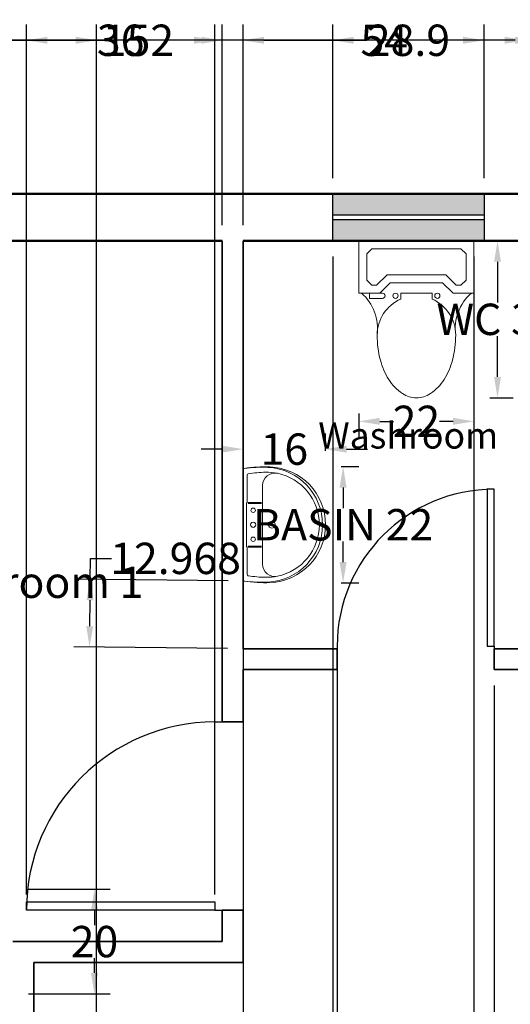
# Model space of a CAD drawing. Units: inches. Extents: x -1285 to -837, y -84 to 552.
# Tile 7 of 10: x -1131 to -1037, y 364 to 552. Entities that reach past the tile are written whole.
import ezdxf

# ---------------------------------------------------------------- set-up
doc = ezdxf.new("R2010")
doc.units = ezdxf.units.IN
doc.header["$MEASUREMENT"] = 0
for name, color, linetype, lineweight in [('A-ANNO-DIMS', 2, 'Continuous', 18), ('A-AREA-IDEN', 7, 'Continuous', 25), ('A-GLAZ-VENT-PATT', 130, 'Continuous', 13), ('Commode', 60, 'Continuous', 18), ('Doors', 34, 'Continuous', 25), ('Inner Wall', 202, 'Continuous', 35), ('Outer Wall', 12, 'Continuous', 50), ('Sink', 33, 'Continuous', 18), ('Ventilators', 130, 'Continuous', 25)]:
    doc.layers.add(name, color=color, linetype=linetype, lineweight=lineweight)
doc.styles.get("Standard").update_dxf_attribs({"font": 'arial.ttf'})
doc.dimstyles.get("Standard").update_dxf_attribs({"dimtxt": 6, "dimasz": 4, "dimexe": 3, "dimexo": 3, "dimgap": 0.09, "dimtad": 0, "dimtih": 1, "dimtoh": 1, "dimdec": 1, "dimzin": 0, "dimdsep": 46, "dimlunit": 3, "dimtxsty": 'Standard', "dimcen": 0.09, "dimadec": 0, "dimazin": 0, "dimtfac": 1, "dimtdec": 1, "dimtofl": 0, "dimtmove": 0, "dimatfit": 3, "dimfxl": 1, "dimtolj": 1, "dimtzin": 0, "dimarcsym": 0})

# ---------------------------------------------------------------- blocks, each defined once
blk = doc.blocks.new('B1')
at = {"color": 0}
for p, q in [((-342.1, -28), (-155.1, -28)), ((-153.6, -35.9), (-153.6, -126.6)), ((-147.1, -24), (-0.5, -24)), ((-147.1, -35.9), (-147.1, -126.6)), ((147.1, -24), (-0.5, -24)), ((147.1, -35.9), (147.1, -126.6)), ((153.6, -35.9), (153.6, -126.6)), ((342.1, -28), (155.1, -28)), ((-0.5, -135), (-272, -135)), ((-0.5, -135), (272.1, -135))]:
    blk.add_line(p, q, dxfattribs=at)
blk.add_lwpolyline([(0, -570, -0.403574), (-399.2, -186.1, -0.04955), (-388.9, -8.4, -0.368901), (-379, 0), (0, 0), (379.1, 0, -0.368901), (388.9, -8.4, -0.04955), (399.3, -186.1, -0.40261)], format="xyb", close=True, dxfattribs=at)
for centre in [(-100.5, -70), (100.6, -70)]:
    blk.add_circle(centre, 15, dxfattribs=at)
for centre, radius, start, end in [((502.9, -129.4), 900, 172.27277, 182.73185), ((437.5, -165.7), 800, 170.69697, 179.27367), ((-342.1, -38), 10, 90, 170.69697), ((-155.1, -24), 4, 270, 323.1301), ((-147.1, -30), 6, 90, 143.1301), ((-0.5, -70), 17.5, 90, 270), ((-0.5, -70), 17.5, 270, 90), ((147.1, -30), 6, 36.8699, 90), ((155.1, -24), 4, 216.8699, 270), ((342.1, -38), 10, 9.30303, 90), ((-437.5, -165.7), 800, 0.72633, 9.30303), ((-502.9, -129.4), 900, 357.26815, 7.72723), ((-272, -220), 85, 90, 191.45253), ((272.1, -220), 85, 348.54747, 90), ((-0.5, -153), 396, 182.79964, 270.07706), ((-0.5, -165), 362, 178.50683, 191.45253), ((0, -200), 23, 90, 270), ((-0.4, -152), 397, 270.055, 357.0633), ((0, -200), 23, 270, 90), ((0.6, -165), 362, 348.54747, 1.49317), ((-0.5, -165), 362, 191.45253, 270.0843), ((-0.4, -163.8), 363.2, 270.06445, 348.39326)]:
    blk.add_arc(centre, radius, start, end, dxfattribs=at)
blk = doc.blocks.new('A$C5EF6120A')
at = {"linetype": 'ByBlock'}
for p, q in [((0, 0.762), (0, 0.508)), ((0, 0.762), (0.5588, 0.762)), ((0.0381, 0.6985), (0.0635, 0.7239)), ((0.0635, 0.7239), (0.4953, 0.7239)), ((0.4953, 0.7239), (0.5207, 0.6985)), ((0.5588, 0.762), (0.5588, 0.508)), ((0.0381, 0.6985), (0.0381, 0.5715)), ((0.5207, 0.6985), (0.5207, 0.5715)), ((0.1366, 0.5969), (0.0858, 0.5461)), ((0.1366, 0.5969), (0.4222, 0.5969)), ((0.4222, 0.5969), (0.473, 0.5461)), ((0.0635, 0.5461), (0.0381, 0.5715)), ((0.0635, 0.5461), (0.0858, 0.5461)), ((0.1524, 0.5588), (0.1016, 0.508)), ((0.1524, 0.5588), (0.4064, 0.5588)), ((0.4064, 0.5588), (0.4572, 0.508)), ((0.4953, 0.5461), (0.473, 0.5461)), ((0.5207, 0.5715), (0.4953, 0.5461)), ((0, 0.508), (0.1016, 0.508)), ((0.0508, 0.508), (0.0508, 0.4826)), ((0.0508, 0.4826), (0.1143, 0.4826)), ((0.1143, 0.508), (0.1016, 0.508)), ((0.2032, 0.508), (0.2032, 0.4794)), ((0.3556, 0.508), (0.2032, 0.508)), ((0.3556, 0.508), (0.3556, 0.4794)), ((0.5588, 0.508), (0.4572, 0.508))]:
    blk.add_line(p, q, dxfattribs=at)
blk.add_lwpolyline([(0.0889, 0.3048, 0.063415), (0.1044, 0.183, 0.076468), (0.1447, 0.0893, 0.107136), (0.2118, 0.0204, 0.147373), (0.2794, 0, 0.147373), (0.347, 0.0204, 0.107136), (0.4141, 0.0893, 0.076468), (0.4544, 0.183, 0.063415), (0.4699, 0.3048, 0.063415)], format="xyb", dxfattribs=at)
for centre in [(0.1778, 0.4953), (0.381, 0.4953)]:
    blk.add_circle(centre, 0.0127, dxfattribs=at)
for centre, radius, start, end in [((-0.1375, 0.3358), 0.2285, 352.2011, 48.911), ((0.2794, 0.3048), 0.1905, 113.5782, 180), ((0.1143, 0.4953), 0.0127, 270, 90), ((0.2794, 0.3048), 0.1905, 0, 66.4218), ((0.6963, 0.3358), 0.2285, 131.089, 187.7989)]:
    blk.add_arc(centre, radius, start, end, dxfattribs=at)
blk = doc.blocks.new('*U3')
for p, q in [((0, 0), (0, -6)), ((40, 0), (40, -6))]:
    blk.add_line(p, q)
blk.add_lwpolyline([(0, 0), (0, 40), (1.75, 40), (1.75, 0)], close=True)
blk.add_arc((0, 0), 40, 0, 90)
blk = doc.blocks.new('*U16')
for p, q in [((0, 0), (0, -6)), ((-40, 0), (-40, -6))]:
    blk.add_line(p, q)
blk.add_lwpolyline([(0, 0), (0, 40), (-1.75, 40), (-1.75, 0)], close=True)
blk.add_arc((0, 0), 40, 90, 180)
blk = doc.blocks.new('*D37')
at = {"layer": 'A-ANNO-DIMS', "color": 0, "lineweight": -2, "transparency": 16777216}
for p, q in [((-1041.37, 509.94), (-1036.87, 509.94)), ((-1039.87, 505.94), (-1039.87, 498.13)), ((-1039.87, 483.93), (-1039.87, 491.74)), ((-1041.37, 479.93), (-1036.87, 479.93))]:
    blk.add_line(p, q, dxfattribs=at)
at = {"layer": 'A-ANNO-DIMS', "color": 0, "transparency": 16777216}
for points in [[(-1040.54, 505.94), (-1039.2, 505.94), (-1039.87, 509.94)], [(-1040.54, 483.93), (-1039.2, 483.93), (-1039.87, 479.93)]]:
    blk.add_solid(points, dxfattribs=at)
at = {"layer": 'Defpoints', "color": 0, "transparency": 16777216}
for p in [(-1044.37, 509.94), (-1039.87, 509.94), (-1044.37, 479.93)]:
    blk.add_point(p, dxfattribs=at)
at = {"layer": 'A-ANNO-DIMS', "color": 0, "transparency": 16777216, "insert": (-1039.87, 494.93), "char_height": 6, "attachment_point": 5}
blk.add_mtext('\\A1;WC 30', dxfattribs=at)
blk = doc.blocks.new('*D38')
at = {"layer": 'A-ANNO-DIMS', "color": 0, "lineweight": -2, "transparency": 16777216}
for p, q in [((-1066.38, 476.93), (-1066.38, 472.42)), ((-1044.37, 476.93), (-1044.37, 472.42)), ((-1062.38, 475.42), (-1059.78, 475.42)), ((-1048.37, 475.42), (-1050.97, 475.42))]:
    blk.add_line(p, q, dxfattribs=at)
at = {"layer": 'A-ANNO-DIMS', "color": 0, "transparency": 16777216}
for points in [[(-1062.38, 476.09), (-1062.38, 474.76), (-1066.38, 475.42)], [(-1048.37, 476.09), (-1048.37, 474.76), (-1044.37, 475.42)]]:
    blk.add_solid(points, dxfattribs=at)
at = {"layer": 'Defpoints', "color": 0, "transparency": 16777216}
for p in [(-1066.38, 479.93), (-1044.37, 479.93), (-1044.37, 475.42)]:
    blk.add_point(p, dxfattribs=at)
at = {"layer": 'A-ANNO-DIMS', "color": 0, "transparency": 16777216, "insert": (-1055.38, 475.42), "char_height": 6, "attachment_point": 5}
blk.add_mtext('\\A1;22', dxfattribs=at)
blk = doc.blocks.new('*D41')
at = {"layer": 'A-ANNO-DIMS', "color": 0, "lineweight": -2, "transparency": 16777216}
for p, q in [((-1069.74, 466.77), (-1066.4, 466.77)), ((-1069.4, 462.77), (-1069.4, 458.84)), ((-1069.4, 448.52), (-1069.4, 452.45)), ((-1069.74, 444.52), (-1066.4, 444.52))]:
    blk.add_line(p, q, dxfattribs=at)
at = {"layer": 'A-ANNO-DIMS', "color": 0, "transparency": 16777216}
for points in [[(-1070.07, 462.77), (-1068.73, 462.77), (-1069.4, 466.77)], [(-1070.07, 448.52), (-1068.73, 448.52), (-1069.4, 444.52)]]:
    blk.add_solid(points, dxfattribs=at)
at = {"layer": 'Defpoints', "color": 0, "transparency": 16777216}
for p in [(-1072.74, 466.77), (-1069.4, 466.77), (-1072.74, 444.52)]:
    blk.add_point(p, dxfattribs=at)
at = {"layer": 'A-ANNO-DIMS', "color": 0, "transparency": 16777216, "insert": (-1069.4, 455.65), "char_height": 6, "attachment_point": 5}
blk.add_mtext('\\A1;BASIN 22', dxfattribs=at)
blk = doc.blocks.new('*D42')
at = {"layer": 'A-ANNO-DIMS', "color": 0, "lineweight": -2, "transparency": 16777216}
for p, q in [((-1088.53, 469.77), (-1088.53, 473.11)), ((-1072.74, 469.77), (-1072.74, 473.11)), ((-1092.53, 470.11), (-1096.53, 470.11)), ((-1068.74, 470.11), (-1064.74, 470.11))]:
    blk.add_line(p, q, dxfattribs=at)
at = {"layer": 'A-ANNO-DIMS', "color": 0, "transparency": 16777216}
for points in [[(-1092.53, 470.77), (-1092.53, 469.44), (-1088.53, 470.11)], [(-1068.74, 470.77), (-1068.74, 469.44), (-1072.74, 470.11)]]:
    blk.add_solid(points, dxfattribs=at)
at = {"layer": 'Defpoints', "color": 0, "transparency": 16777216}
for p in [(-1088.53, 470.11), (-1088.53, 466.77), (-1072.74, 466.77)]:
    blk.add_point(p, dxfattribs=at)
at = {"layer": 'A-ANNO-DIMS', "color": 0, "transparency": 16777216, "insert": (-1080.63, 470.11), "char_height": 6, "attachment_point": 5}
blk.add_mtext('\\A1;16', dxfattribs=at)
blk = doc.blocks.new('*D60')
at = {"layer": 'A-ANNO-DIMS', "color": 0, "lineweight": -2, "transparency": 16777216}
for p, q in [((-1129.53, 385.94), (-1113.93, 385.94)), ((-1116.93, 381.94), (-1116.93, 379.09)), ((-1116.93, 369.94), (-1116.93, 372.79)), ((-1129.53, 365.94), (-1113.93, 365.94))]:
    blk.add_line(p, q, dxfattribs=at)
at = {"layer": 'A-ANNO-DIMS', "color": 0, "transparency": 16777216}
for points in [[(-1117.6, 381.94), (-1116.26, 381.94), (-1116.93, 385.94)], [(-1117.6, 369.94), (-1116.26, 369.94), (-1116.93, 365.94)]]:
    blk.add_solid(points, dxfattribs=at)
at = {"layer": 'Defpoints', "color": 0, "transparency": 16777216}
for p in [(-1132.53, 385.94), (-1116.93, 385.94), (-1132.53, 365.94)]:
    blk.add_point(p, dxfattribs=at)
at = {"layer": 'A-ANNO-DIMS', "color": 0, "transparency": 16777216, "insert": (-1116.93, 375.94), "char_height": 6, "attachment_point": 5}
blk.add_mtext('\\A1;20', dxfattribs=at)
blk = doc.blocks.new('*D71')
at = {"layer": 'A-ANNO-DIMS', "color": 0, "lineweight": -2, "transparency": 16777216}
for p, q in [((-1236.53, 512.94), (-1236.53, 551.29)), ((-1092.53, 512.94), (-1092.53, 551.29)), ((-1232.53, 548.29), (-1170.95, 548.29)), ((-1096.53, 548.29), (-1158.11, 548.29))]:
    blk.add_line(p, q, dxfattribs=at)
at = {"layer": 'A-ANNO-DIMS', "color": 0, "transparency": 16777216}
for points in [[(-1232.53, 548.96), (-1232.53, 547.62), (-1236.53, 548.29)], [(-1096.53, 548.96), (-1096.53, 547.62), (-1092.53, 548.29)]]:
    blk.add_solid(points, dxfattribs=at)
at = {"layer": 'Defpoints', "color": 0, "transparency": 16777216}
for p in [(-1092.53, 548.29), (-1236.53, 509.94), (-1092.53, 509.94)]:
    blk.add_point(p, dxfattribs=at)
at = {"layer": 'A-ANNO-DIMS', "color": 0, "transparency": 16777216, "insert": (-1164.53, 548.29), "char_height": 6, "attachment_point": 5}
blk.add_mtext('\\A1;144', dxfattribs=at)
blk = doc.blocks.new('*D72')
at = {"layer": 'A-ANNO-DIMS', "color": 0, "lineweight": -2, "transparency": 16777216}
for p, q in [((-1088.53, 512.94), (-1088.53, 551.29)), ((-1034.53, 512.94), (-1034.53, 551.29)), ((-1084.53, 548.29), (-1065.9, 548.29)), ((-1038.53, 548.29), (-1057.15, 548.29))]:
    blk.add_line(p, q, dxfattribs=at)
at = {"layer": 'A-ANNO-DIMS', "color": 0, "transparency": 16777216}
for points in [[(-1084.53, 548.96), (-1084.53, 547.62), (-1088.53, 548.29)], [(-1038.53, 548.96), (-1038.53, 547.62), (-1034.53, 548.29)]]:
    blk.add_solid(points, dxfattribs=at)
at = {"layer": 'Defpoints', "color": 0, "transparency": 16777216}
for p in [(-1034.53, 548.29), (-1088.53, 509.94), (-1034.53, 509.94)]:
    blk.add_point(p, dxfattribs=at)
at = {"layer": 'A-ANNO-DIMS', "color": 0, "transparency": 16777216, "insert": (-1061.53, 548.29), "char_height": 6, "attachment_point": 5}
blk.add_mtext('\\A1;54', dxfattribs=at)
blk = doc.blocks.new('*D78')
at = {"layer": 'A-ANNO-DIMS', "color": 0, "lineweight": -2, "transparency": 16777216}
for p, q in [((-1236.53, 162.94), (-1236.53, 551.29)), ((-1116.53, 162.94), (-1116.53, 551.29)), ((-1232.53, 548.29), (-1182.96, 548.29)), ((-1120.53, 548.29), (-1170.1, 548.29))]:
    blk.add_line(p, q, dxfattribs=at)
at = {"layer": 'A-ANNO-DIMS', "color": 0, "transparency": 16777216}
for points in [[(-1232.53, 548.96), (-1232.53, 547.62), (-1236.53, 548.29)], [(-1120.53, 548.96), (-1120.53, 547.62), (-1116.53, 548.29)]]:
    blk.add_solid(points, dxfattribs=at)
at = {"layer": 'Defpoints', "color": 0, "transparency": 16777216}
for p in [(-1116.53, 548.29), (-1236.53, 159.94), (-1116.53, 159.94)]:
    blk.add_point(p, dxfattribs=at)
at = {"layer": 'A-ANNO-DIMS', "color": 0, "transparency": 16777216, "insert": (-1176.53, 548.29), "char_height": 6, "attachment_point": 5}
blk.add_mtext('\\A1;120', dxfattribs=at)
blk = doc.blocks.new('*D80')
at = {"layer": 'A-ANNO-DIMS', "color": 0, "lineweight": -2, "transparency": 16777216}
for p, q in [((-1184.53, -13.66), (-1184.53, 551.29)), ((-1032.53, -13.66), (-1032.53, 551.29)), ((-1180.53, 548.29), (-1114.94, 548.29)), ((-1036.53, 548.29), (-1102.12, 548.29))]:
    blk.add_line(p, q, dxfattribs=at)
at = {"layer": 'A-ANNO-DIMS', "color": 0, "transparency": 16777216}
for points in [[(-1180.53, 548.96), (-1180.53, 547.62), (-1184.53, 548.29)], [(-1036.53, 548.96), (-1036.53, 547.62), (-1032.53, 548.29)]]:
    blk.add_solid(points, dxfattribs=at)
at = {"layer": 'Defpoints', "color": 0, "transparency": 16777216}
for p in [(-1032.53, 548.29), (-1184.53, -16.66), (-1032.53, -16.66)]:
    blk.add_point(p, dxfattribs=at)
at = {"layer": 'A-ANNO-DIMS', "color": 0, "transparency": 16777216, "insert": (-1108.53, 548.29), "char_height": 6, "attachment_point": 5}
blk.add_mtext('\\A1;152', dxfattribs=at)
blk = doc.blocks.new('*D87')
at = {"layer": 'A-ANNO-DIMS', "color": 0, "lineweight": -2, "transparency": 16777216}
for p, q in [((-1070.53, 424.94), (-1070.53, -83.53)), ((-1040.53, 424.94), (-1040.53, -83.53)), ((-1066.53, -80.53), (-1059.9, -80.53)), ((-1044.53, -80.53), (-1051.15, -80.53))]:
    blk.add_line(p, q, dxfattribs=at)
at = {"layer": 'A-ANNO-DIMS', "color": 0, "transparency": 16777216}
for points in [[(-1066.53, -79.86), (-1066.53, -81.2), (-1070.53, -80.53)], [(-1044.53, -79.86), (-1044.53, -81.2), (-1040.53, -80.53)]]:
    blk.add_solid(points, dxfattribs=at)
at = {"layer": 'Defpoints', "color": 0, "transparency": 16777216}
for p in [(-1070.53, 427.94), (-1040.53, 427.94), (-1040.53, -80.53)]:
    blk.add_point(p, dxfattribs=at)
at = {"layer": 'A-ANNO-DIMS', "color": 0, "transparency": 16777216, "insert": (-1055.53, -80.53), "char_height": 6, "attachment_point": 5}
blk.add_mtext('\\A1;30', dxfattribs=at)
blk = doc.blocks.new('*D89')
at = {"layer": 'A-ANNO-DIMS', "color": 0, "lineweight": -2, "transparency": 16777216}
for p, q in [((-1071.35, 521.94), (-1071.35, 551.29)), ((-1042.45, 521.94), (-1042.45, 551.29)), ((-1067.35, 548.29), (-1064.84, 548.29)), ((-1046.45, 548.29), (-1048.96, 548.29))]:
    blk.add_line(p, q, dxfattribs=at)
at = {"layer": 'A-ANNO-DIMS', "color": 0, "transparency": 16777216}
for points in [[(-1067.35, 548.96), (-1067.35, 547.62), (-1071.35, 548.29)], [(-1046.45, 548.96), (-1046.45, 547.62), (-1042.45, 548.29)]]:
    blk.add_solid(points, dxfattribs=at)
at = {"layer": 'Defpoints', "color": 0, "transparency": 16777216}
for p in [(-1042.45, 548.29), (-1071.35, 518.94), (-1042.45, 518.94)]:
    blk.add_point(p, dxfattribs=at)
at = {"layer": 'A-ANNO-DIMS', "color": 0, "transparency": 16777216, "insert": (-1056.9, 548.29), "char_height": 6, "attachment_point": 5}
blk.add_mtext('\\A1;28.9', dxfattribs=at)
blk = doc.blocks.new('*D90')
at = {"layer": 'A-ANNO-DIMS', "color": 0, "lineweight": -2, "transparency": 16777216}
for p, q in [((-1129.93, 384.94), (-1129.93, 551.29)), ((-1093.93, 384.94), (-1093.93, 551.29)), ((-1125.93, 548.29), (-1116.31, 548.29)), ((-1097.93, 548.29), (-1107.55, 548.29))]:
    blk.add_line(p, q, dxfattribs=at)
at = {"layer": 'A-ANNO-DIMS', "color": 0, "transparency": 16777216}
for points in [[(-1125.93, 548.96), (-1125.93, 547.62), (-1129.93, 548.29)], [(-1097.93, 548.96), (-1097.93, 547.62), (-1093.93, 548.29)]]:
    blk.add_solid(points, dxfattribs=at)
at = {"layer": 'Defpoints', "color": 0, "transparency": 16777216}
for p in [(-1093.93, 548.29), (-1129.93, 381.94), (-1093.93, 381.94)]:
    blk.add_point(p, dxfattribs=at)
at = {"layer": 'A-ANNO-DIMS', "color": 0, "transparency": 16777216, "insert": (-1111.93, 548.29), "char_height": 6, "attachment_point": 5}
blk.add_mtext('\\A1;36', dxfattribs=at)
blk = doc.blocks.new('*D103')
at = {"layer": 'A-ANNO-DIMS', "color": 0, "lineweight": -2, "transparency": 16777216}
for p, q in [((-1088.53, 506.94), (-1088.53, -83.53)), ((-1071.35, 506.94), (-1071.35, -83.53)), ((-1084.53, -80.53), (-1075.35, -80.53)), ((-1071.35, -80.53), (-1067.35, -80.53))]:
    blk.add_line(p, q, dxfattribs=at)
at = {"layer": 'A-ANNO-DIMS', "color": 0, "transparency": 16777216}
for points in [[(-1084.53, -79.86), (-1084.53, -81.2), (-1088.53, -80.53)], [(-1075.35, -79.86), (-1075.35, -81.2), (-1071.35, -80.53)]]:
    blk.add_solid(points, dxfattribs=at)
at = {"layer": 'Defpoints', "color": 0, "transparency": 16777216}
for p in [(-1088.53, 509.94), (-1071.35, 509.94), (-1071.35, -80.53)]:
    blk.add_point(p, dxfattribs=at)
at = {"layer": 'A-ANNO-DIMS', "color": 0, "transparency": 16777216, "insert": (-1057.41, -80.53), "char_height": 6, "attachment_point": 5}
blk.add_mtext('\\A1;17.18', dxfattribs=at)
blk = doc.blocks.new('*D104')
at = {"layer": 'A-ANNO-DIMS', "color": 0, "lineweight": -2, "transparency": 16777216}
for p, q in [((-1044.37, 506.94), (-1044.37, -83.53)), ((-1034.53, 506.94), (-1034.53, -83.53)), ((-1040.37, -80.53), (-1038.53, -80.53)), ((-1034.53, -80.53), (-1030.53, -80.53))]:
    blk.add_line(p, q, dxfattribs=at)
at = {"layer": 'A-ANNO-DIMS', "color": 0, "transparency": 16777216}
for points in [[(-1040.37, -79.86), (-1040.37, -81.2), (-1044.37, -80.53)], [(-1038.53, -79.86), (-1038.53, -81.2), (-1034.53, -80.53)]]:
    blk.add_solid(points, dxfattribs=at)
at = {"layer": 'Defpoints', "color": 0, "transparency": 16777216}
for p in [(-1044.37, 509.94), (-1034.53, 509.94), (-1034.53, -80.53)]:
    blk.add_point(p, dxfattribs=at)
at = {"layer": 'A-ANNO-DIMS', "color": 0, "transparency": 16777216, "insert": (-1022.66, -80.53), "char_height": 6, "attachment_point": 5}
blk.add_mtext('\\A1;9.84', dxfattribs=at)
blk = doc.blocks.new('*D105')
at = {"layer": 'A-ANNO-DIMS', "color": 0, "lineweight": -2, "transparency": 16777216}
for p, q in [((-1088.53, 428.94), (-1088.53, -83.53)), ((-1070.53, 428.94), (-1070.53, -83.53)), ((-1084.53, -80.53), (-1083.64, -80.53)), ((-1074.53, -80.53), (-1075.42, -80.53))]:
    blk.add_line(p, q, dxfattribs=at)
at = {"layer": 'A-ANNO-DIMS', "color": 0, "transparency": 16777216}
for points in [[(-1084.53, -79.86), (-1084.53, -81.2), (-1088.53, -80.53)], [(-1074.53, -79.86), (-1074.53, -81.2), (-1070.53, -80.53)]]:
    blk.add_solid(points, dxfattribs=at)
at = {"layer": 'Defpoints', "color": 0, "transparency": 16777216}
for p in [(-1088.53, 431.94), (-1070.53, 431.94), (-1070.53, -80.53)]:
    blk.add_point(p, dxfattribs=at)
at = {"layer": 'A-ANNO-DIMS', "color": 0, "transparency": 16777216, "insert": (-1079.53, -80.53), "char_height": 6, "attachment_point": 5}
blk.add_mtext('\\A1;18', dxfattribs=at)
blk = doc.blocks.new('*D106')
at = {"layer": 'A-ANNO-DIMS', "color": 0, "lineweight": -2, "transparency": 16777216}
for p, q in [((-1274.88, 365.94), (-1274.88, 369.94)), ((-1274.88, 369.94), (-1270.88, 369.94)), ((-983.53, 361.94), (-1277.88, 361.94)), ((-983.53, 355.94), (-1277.88, 355.94)), ((-1274.88, 351.94), (-1274.88, 347.94))]:
    blk.add_line(p, q, dxfattribs=at)
at = {"layer": 'A-ANNO-DIMS', "color": 0, "transparency": 16777216}
for points in [[(-1275.55, 365.94), (-1274.21, 365.94), (-1274.88, 361.94)], [(-1275.55, 351.94), (-1274.21, 351.94), (-1274.88, 355.94)]]:
    blk.add_solid(points, dxfattribs=at)
at = {"layer": 'Defpoints', "color": 0, "transparency": 16777216}
for p in [(-1274.88, 361.94), (-980.53, 361.94), (-980.53, 355.94)]:
    blk.add_point(p, dxfattribs=at)
at = {"layer": 'A-ANNO-DIMS', "color": 0, "transparency": 16777216, "insert": (-1268.81, 369.94), "char_height": 6, "attachment_point": 5}
blk.add_mtext('\\A1;6', dxfattribs=at)
blk = doc.blocks.new('*D118')
at = {"layer": 'A-ANNO-DIMS', "color": 0, "lineweight": -2, "transparency": 16777216}
for p, q in [((-1117.74, 445.22), (-1117.69, 449.22)), ((-1117.69, 449.22), (-1113.69, 449.22)), ((-1091.39, 444.94), (-1120.74, 445.26)), ((-1117.83, 436.26), (-1117.78, 441.22)), ((-1091.53, 431.97), (-1120.88, 432.29))]:
    blk.add_line(p, q, dxfattribs=at)
at = {"layer": 'A-ANNO-DIMS', "color": 0, "transparency": 16777216}
for points in [[(-1118.45, 441.23), (-1117.11, 441.22), (-1117.74, 445.22)], [(-1118.5, 436.26), (-1117.17, 436.25), (-1117.88, 432.26)]]:
    blk.add_solid(points, dxfattribs=at)
at = {"layer": 'Defpoints', "color": 0, "transparency": 16777216}
for p in [(-1117.74, 445.22), (-1088.39, 444.91), (-1088.53, 431.94)]:
    blk.add_point(p, dxfattribs=at)
at = {"layer": 'A-ANNO-DIMS', "color": 0, "transparency": 16777216, "insert": (-1101.43, 449.22), "char_height": 6, "attachment_point": 5}
blk.add_mtext('\\A1;12.968', dxfattribs=at)

msp = doc.modelspace()

# ---------------------------------------------------------------- hatches: boundary and pattern name
at = {"layer": 'A-GLAZ-VENT-PATT'}
h = msp.add_hatch(color=256, dxfattribs=at)
h.dxf.hatch_style = 1
h.paths.add_polyline_path([(-1042.4483, 518.9392), (-1071.3483, 518.9392), (-1071.3483, 514.9392), (-1042.4483, 514.9392)])
h.paths.add_polyline_path([(-1042.4483, 513.9392), (-1071.3483, 513.9392), (-1071.3483, 509.9392), (-1042.4483, 509.9392)])

# ---------------------------------------------------------------- linework, layer by layer
at = {"layer": 'Inner Wall'}
for p, q in [((-1092.5299, 509.9392), (-1092.5299, 417.9392)), ((-1088.5299, 509.9392), (-1088.5299, 431.9392)), ((-1088.5299, 431.9392), (-1070.5299, 431.9392)), ((-1070.5299, 431.9392), (-1070.5299, 427.9392)), ((-1040.5299, 431.9392), (-1040.5299, 427.9392)), ((-1040.5299, 431.9392), (-1034.5299, 431.9392)), ((-1088.5299, 427.9392), (-1070.5299, 427.9392)), ((-1088.5299, 427.9392), (-1088.5299, 417.9392)), ((-1040.5299, 427.9392), (-1034.5299, 427.9392)), ((-1092.5299, 417.9392), (-1088.5299, 417.9392)), ((-1092.5299, 381.9392), (-1088.5299, 381.9392)), ((-1092.5299, 381.9392), (-1092.5299, 375.9392)), ((-1088.5299, 381.9392), (-1088.5299, 371.9392)), ((-1132.5299, 375.9392), (-1092.5299, 375.9392)), ((-1128.5299, 371.9392), (-1088.5299, 371.9392)), ((-1128.5299, 371.9392), (-1128.5299, 361.9392))]:
    msp.add_line(p, q, dxfattribs=at)
at = {"layer": 'Outer Wall'}
for p, q in [((-1245.5299, 518.9392), (-877.5299, 518.9392)), ((-1236.5299, 509.9392), (-1092.5299, 509.9392)), ((-1088.5299, 509.9392), (-1034.5299, 509.9392))]:
    msp.add_line(p, q, dxfattribs=at)
at = {"layer": 'Ventilators'}
for p, q in [((-1071.3483, 514.9392), (-1042.4483, 514.9392)), ((-1042.4483, 513.9392), (-1071.3483, 513.9392))]:
    msp.add_line(p, q, dxfattribs=at)
msp.add_lwpolyline([(-1042.4483, 518.9392), (-1042.4483, 509.9392), (-1071.3483, 509.9392), (-1071.3483, 518.9392)], close=True, dxfattribs=at)

# ---------------------------------------------------------------- block references
at = {"layer": 'Commode', "xscale": 39.38712823985619, "yscale": 39.38712823985619, "zscale": 39.38712823985619}
msp.add_blockref('A$C5EF6120A', (-1066.3798, 479.9262), dxfattribs=at)
at = {"layer": 'Doors', "xscale": 0.75, "yscale": 0.75, "zscale": 0.75}
msp.add_blockref('*U16', (-1040.5299, 432.4392), dxfattribs=at)
at = {"layer": 'Doors', "xscale": 0.9, "yscale": 0.9, "zscale": 0.9, "rotation": 90}
msp.add_blockref('*U3', (-1093.9299, 381.9392), dxfattribs=at)
at = {"layer": 'Sink', "xscale": 0.0276945458005416, "yscale": 0.0276945458005416, "zscale": 0.0276945458005416, "rotation": 89.99999999999999}
msp.add_blockref('B1', (-1088.5299, 455.6451), dxfattribs=at)

# ---------------------------------------------------------------- texts
at = {"layer": 'A-AREA-IDEN', "attachment_point": 1}
for s, insert, char_height in [('Washroom', (-1074.1396, 475.2155), 5), ('Bedroom 1', (-1149.6203, 447.6499), 6)]:
    msp.add_mtext_dynamic_manual_height_columns(s, width=68.784729, gutter_width=1, heights=[0], dxfattribs=dict(at, insert=insert, char_height=char_height))

# ---------------------------------------------------------------- dimensions: what is measured, and where the dimension line sits
at = {"layer": 'A-ANNO-DIMS'}
for base, p1, p2, override, picture, middle in [((-1092.5299, 548.2892), (-1236.5299, 509.9392), (-1092.5299, 509.9392), {"dimdec": 0, "dimlfac": 1, "dimrnd": 0, "dimzin": 0, "dimdsep": 46, "dimlunit": 2}, '*D71', (-1164.5299, 548.2892)), ((-1116.5299, 548.2892), (-1236.5299, 159.9392), (-1116.5299, 159.9392), {"dimdec": 0, "dimlfac": 1, "dimrnd": 0, "dimzin": 0, "dimdsep": 46, "dimlunit": 2}, '*D78', (-1176.5299, 548.2892)), ((-1032.5299, 548.2892), (-1184.5299, -16.6608), (-1032.5299, -16.6608), {"dimdec": 0, "dimlfac": 1, "dimrnd": 0, "dimzin": 0, "dimdsep": 46, "dimlunit": 2}, '*D80', (-1108.5299, 548.2892)), ((-1093.9299, 548.2892), (-1129.9299, 381.9392), (-1093.9299, 381.9392), {"dimdec": 0, "dimlfac": 1, "dimrnd": 0, "dimzin": 0, "dimdsep": 46, "dimlunit": 2}, '*D90', (-1111.9299, 548.2892)), ((-1034.5299, 548.2892), (-1088.5299, 509.9392), (-1034.5299, 509.9392), {"dimdec": 0, "dimlfac": 1, "dimrnd": 0, "dimzin": 0, "dimdsep": 46, "dimlunit": 2}, '*D72', (-1061.5299, 548.2892)), ((-1042.4483, 548.2892), (-1071.3483, 518.9392), (-1042.4483, 518.9392), {"dimdec": 1, "dimlfac": 1, "dimrnd": 0, "dimzin": 0, "dimdsep": 46, "dimlunit": 2}, '*D89', (-1056.8983, 548.2892)), ((-1071.3483, -80.5308), (-1088.5299, 509.9392), (-1071.3483, 509.9392), {"dimdec": 2, "dimlfac": 1, "dimrnd": 0, "dimzin": 0, "dimdsep": 46, "dimlunit": 2}, '*D103', (-1057.4111, -80.5308)), ((-1034.5299, -80.5308), (-1044.3703, 509.9392), (-1034.5299, 509.9392), {"dimdec": 2, "dimlfac": 1, "dimrnd": 0, "dimzin": 0, "dimdsep": 46, "dimlunit": 2}, '*D104', (-1022.6595, -80.5308)), ((-1044.3703, 475.4243), (-1066.3798, 479.9262), (-1044.3703, 479.9262), {"dimdec": 0, "dimlfac": 1, "dimrnd": 0, "dimzin": 0, "dimdsep": 46, "dimlunit": 2}, '*D38', (-1055.375, 475.4243)), ((-1070.5299, -80.5308), (-1088.5299, 431.9392), (-1070.5299, 431.9392), {"dimdec": 0, "dimlfac": 1, "dimrnd": 0, "dimzin": 0, "dimdsep": 46, "dimlunit": 2}, '*D105', (-1079.5299, -80.5308)), ((-1040.5299, -80.5308), (-1070.5299, 427.9392), (-1040.5299, 427.9392), {"dimdec": 0, "dimlfac": 1, "dimrnd": 0, "dimzin": 0, "dimdsep": 46, "dimlunit": 2}, '*D87', (-1055.5299, -80.5308))]:
    dim = msp.add_linear_dim(base=base, p1=p1, p2=p2, dimstyle='Standard', override=override, dxfattribs=at)
    dim.commit()
    dim.dimension.update_dxf_attribs({"geometry": picture, "text_midpoint": middle})
for base, p1, p2, text, picture, middle in [((-1039.8683, 509.9392), (-1044.3703, 479.9262), (-1044.3703, 509.9392), 'WC <>', '*D37', (-1039.8683, 494.9327)), ((-1069.3986, 466.7703), (-1072.736, 444.5208), (-1072.736, 466.7703), 'BASIN <>', '*D41', (-1069.3986, 455.6456))]:
    dim = msp.add_linear_dim(base=base, p1=p1, p2=p2, angle=90, text=text, dimstyle='Standard', override={"dimdec": 0, "dimlfac": 1, "dimrnd": 0, "dimzin": 0, "dimdsep": 46, "dimlunit": 2}, dxfattribs=at)
    dim.commit()
    dim.dimension.update_dxf_attribs({"geometry": picture, "text_midpoint": middle})
for base, p1, p2, angle, override, picture, middle in [((-1088.5299, 470.1078), (-1072.736, 466.7703), (-1088.5299, 466.7703), 180, {"dimdec": 0, "dimlfac": 1, "dimrnd": 0, "dimzin": 0, "dimdsep": 46, "dimlunit": 2}, '*D42', (-1080.633, 470.1078)), ((-1117.73781, 445.22458), (-1088.52987, 431.93924), (-1088.38952, 444.90695), 89.379941, {"dimdec": 3, "dimlfac": 1, "dimrnd": 0, "dimzin": 0, "dimdsep": 46, "dimlunit": 2}, '*D118', (-1101.42648, 449.22434)), ((-1116.9299, 385.9392), (-1132.5299, 365.9392), (-1132.5299, 385.9392), 90, {"dimdec": 0, "dimlfac": 1, "dimrnd": 0, "dimzin": 0, "dimdsep": 46, "dimlunit": 2}, '*D60', (-1116.9299, 375.9392)), ((-1274.8799, 361.9392), (-980.5299, 355.9392), (-980.5299, 361.9392), 90, {"dimdec": 0, "dimlfac": 1, "dimrnd": 0, "dimzin": 0, "dimdsep": 46, "dimlunit": 2}, '*D106', (-1268.809, 369.9392))]:
    dim = msp.add_linear_dim(base=base, p1=p1, p2=p2, angle=angle, dimstyle='Standard', override=override, dxfattribs=at)
    dim.commit()
    dim.dimension.update_dxf_attribs({"geometry": picture, "text_midpoint": middle})

doc.saveas('drawing.dxf')
